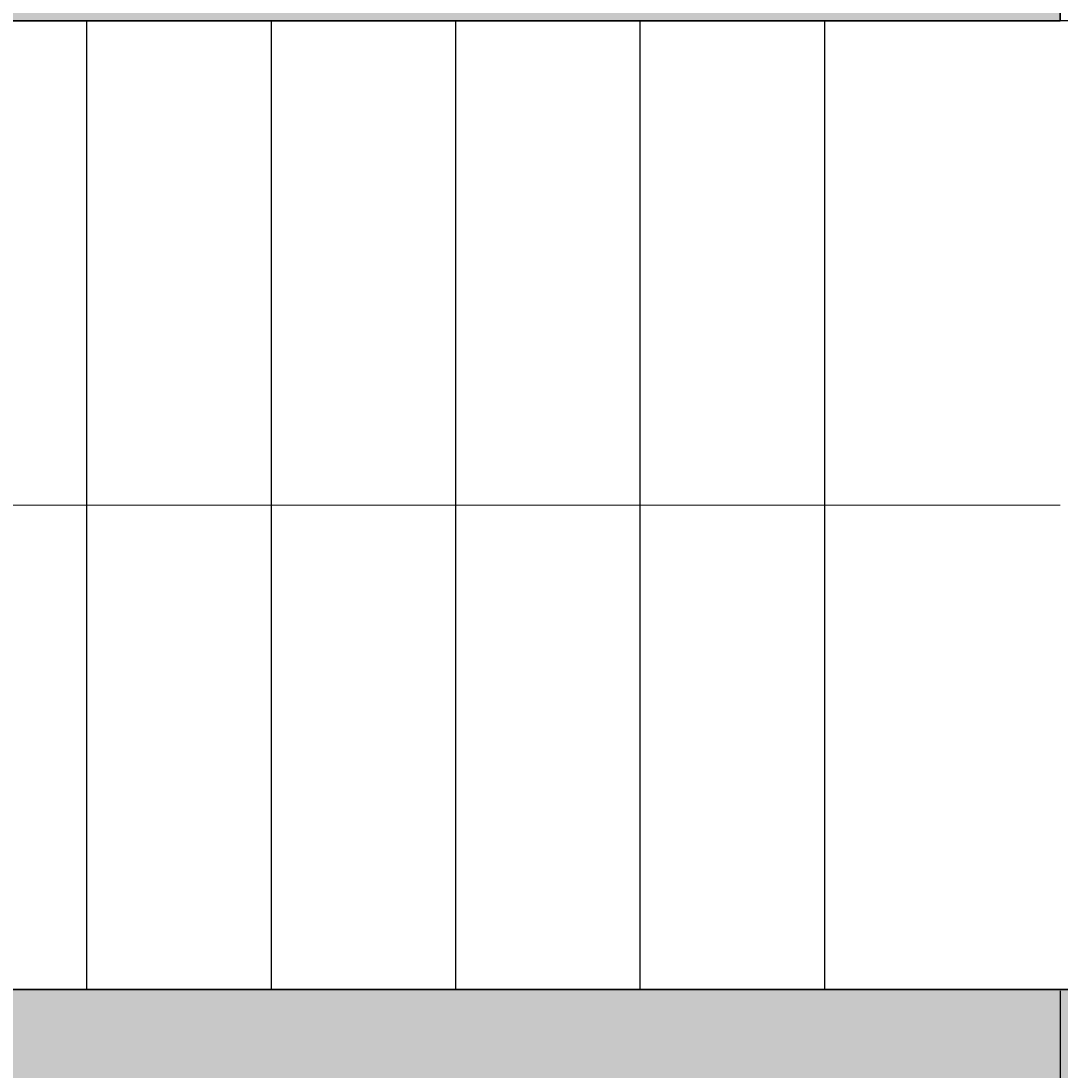
# Model space of a CAD drawing. Units: inches. Extents: x 1998 to 2588, y 1139 to 1977.
# Tile 93 of 134: x 2453 to 2498, y 1477 to 1523. Entities that reach past the tile are written whole.
import ezdxf

# ---------------------------------------------------------------- set-up
doc = ezdxf.new("R2010")
doc.units = ezdxf.units.IN
for name, color, linetype, lineweight in [('A-ANNO-DIMS', 2, 'Continuous', 18), ('A-ANNO-SYMB', 7, 'Continuous', 18), ('A-FLOR-EVTR', 7, 'Continuous', 35), ('A-FLOR-STRS', 7, 'Continuous', 25), ('A-WALL-PATT', 252, 'Continuous', 13), ('WALL', 200, 'Continuous', 35)]:
    doc.layers.add(name, color=color, linetype=linetype, lineweight=lineweight)
doc.styles.get("Standard").update_dxf_attribs({"font": 'arial.ttf'})
doc.dimstyles.get("Standard").update_dxf_attribs({"dimtxt": 0.18, "dimasz": 0.18, "dimexe": 0.18, "dimexo": 0.0625, "dimgap": 0.09, "dimtad": 0, "dimtih": 1, "dimtoh": 1, "dimdec": 4, "dimzin": 0, "dimdsep": 46, "dimtxsty": 'Standard', "dimcen": 0.09, "dimadec": 0, "dimazin": 0, "dimtfac": 1, "dimtdec": 4, "dimtofl": 0, "dimtmove": 0, "dimatfit": 3, "dimfxl": 1, "dimtolj": 1, "dimtzin": 0, "dimarcsym": 0})

# ---------------------------------------------------------------- blocks, each defined once
blk = doc.blocks.new('*D24')
at = {"layer": 'A-ANNO-DIMS', "color": 0, "lineweight": -2, "transparency": 16777216}
for p, q in [((2398.535, 1911.232), (2588.309, 1911.232)), ((2588.129, 1911.052), (2588.129, 1570.164)), ((2588.129, 1228.912), (2588.129, 1569.8)), ((2527.535, 1228.732), (2588.309, 1228.732))]:
    blk.add_line(p, q, dxfattribs=at)
at = {"layer": 'A-ANNO-DIMS', "color": 0, "transparency": 16777216}
for points in [[(2588.099, 1911.052), (2588.159, 1911.052), (2588.129, 1911.232)], [(2588.099, 1228.912), (2588.159, 1228.912), (2588.129, 1228.732)]]:
    blk.add_solid(points, dxfattribs=at)
at = {"layer": 'Defpoints', "color": 0, "transparency": 16777216}
for p in [(2398.473, 1911.232), (2588.129, 1911.232), (2527.473, 1228.732)]:
    blk.add_point(p, dxfattribs=at)
at = {"layer": 'A-ANNO-DIMS', "color": 0, "transparency": 16777216, "insert": (2588.129, 1569.982), "char_height": 0.18, "attachment_point": 5}
blk.add_mtext('\\A1;682.5', dxfattribs=at)
blk = doc.blocks.new('*D33')
at = {"layer": 'A-ANNO-DIMS', "color": 0, "lineweight": -2, "transparency": 16777216}
for p, q in [((2407.973, 1480.67), (2407.973, 1138.602)), ((2498.179, 1480.67), (2498.179, 1138.602)), ((2408.153, 1138.782), (2452.753, 1138.782)), ((2497.999, 1138.782), (2453.399, 1138.782))]:
    blk.add_line(p, q, dxfattribs=at)
at = {"layer": 'A-ANNO-DIMS', "color": 0, "transparency": 16777216}
for points in [[(2408.153, 1138.812), (2408.153, 1138.752), (2407.973, 1138.782)], [(2497.999, 1138.812), (2497.999, 1138.752), (2498.179, 1138.782)]]:
    blk.add_solid(points, dxfattribs=at)
at = {"layer": 'Defpoints', "color": 0, "transparency": 16777216}
for p in [(2407.973, 1480.732), (2498.179, 1480.732), (2498.179, 1138.782)]:
    blk.add_point(p, dxfattribs=at)
at = {"layer": 'A-ANNO-DIMS', "color": 0, "transparency": 16777216, "insert": (2453.076, 1138.782), "char_height": 0.18, "attachment_point": 5}
blk.add_mtext('\\A1;90.2', dxfattribs=at)

msp = doc.modelspace()

# ---------------------------------------------------------------- hatches: boundary and pattern name
at = {"layer": 'A-WALL-PATT'}
h = msp.add_hatch(color=256, dxfattribs=at)
h.dxf.hatch_style = 1
h.paths.add_polyline_path([(2527.4729, 1362.2324), (2510.9729, 1362.2324), (2510.9729, 1357.7324), (2518.4729, 1357.7324), (2518.4729, 1237.7324), (2503.1458, 1237.7324), (2503.1458, 1228.7324), (2527.4729, 1228.7324)])
h.paths.add_polyline_path([(2490.5682, 1362.2324), (2398.4729, 1362.2324), (2398.4729, 1357.7324), (2490.5682, 1357.7324)])
h.paths.add_polyline_path([(2224.9729, 1264.7324), (2222.9729, 1264.7324), (2222.9729, 1232.4125), (2341.4729, 1232.4125), (2341.4729, 1234.4125), (2224.9729, 1234.4125)])
h.paths.add_polyline_path([(2334.5332, 1273.7324), (2264.7638, 1273.7324), (2264.7638, 1269.5611, -0.043659), (2264.3413, 1264.7324), (2334.5332, 1264.7324)])
h.paths.add_polyline_path([(2236.9551, 1273.7324), (2234.4125, 1273.7324), (2234.4125, 1264.7324), (2236.9551, 1264.7324), (2236.9551, 1269.5611)])
h.paths.add_polyline_path([(2222.9729, 1293.2324), (2096.9729, 1293.2324), (2096.9729, 1345.0966), (2087.9729, 1345.0966), (2087.9729, 1284.2324), (2222.9729, 1284.2324), (2222.9729, 1285.137)])
h.paths.add_polyline_path([(2096.9729, 1458.7927), (2087.9729, 1458.7927), (2087.9729, 1417.7324), (2087.9729, 1413.2324), (2096.9729, 1413.2324), (2096.9729, 1417.7324)])
h.paths.add_polyline_path([(2096.9729, 1413.2324), (2087.9729, 1413.2324), (2087.9729, 1365.5012), (2096.9729, 1365.5012), (2096.9729, 1369.3358)])
h.paths.add_polyline_path([(2186.2943, 1417.7324), (2138.6074, 1417.7324), (2096.9729, 1417.7324), (2096.9729, 1413.2324), (2138.6074, 1413.2324), (2186.2943, 1413.2324)])
h.paths.add_polyline_path([(2181.4729, 1465.7324), (2176.9729, 1465.7324), (2176.9729, 1451.6434), (2181.4729, 1451.6434)])
h.paths.add_polyline_path([(2181.4729, 1422.1664), (2176.9729, 1422.1664), (2176.9729, 1417.7324), (2181.4729, 1417.7324)])
h.paths.add_polyline_path([(2063.9729, 1465.7324), (2087.9729, 1465.7324), (2087.9729, 1470.2324), (2059.4729, 1470.2324), (2059.4729, 1413.2324), (2087.9729, 1413.2324), (2087.9729, 1417.7324), (2063.9729, 1417.7324)])
h.paths.add_polyline_path([(2181.4729, 1755.2324), (2176.9729, 1755.2324), (2176.9729, 1748.6798), (2177.0513, 1748.6798), (2181.4729, 1748.6798)])
h.paths.add_polyline_path([(2227.4729, 1707.2324), (2220.4647, 1707.2324), (2220.4647, 1702.7324), (2222.9729, 1702.7324), (2222.9729, 1604.637), (2227.4729, 1604.637)])
h.paths.add_polyline_path([(2114.9729, 1702.7324), (2105.9729, 1702.7324), (2105.9729, 1628.4781, -0.0318759), (2110.1012, 1628.7416), (2114.9729, 1628.7416)])
h.paths.add_polyline_path([(2345.9729, 1739.3278), (2341.4729, 1739.3278), (2341.4729, 1647.5211), (2345.9729, 1647.5211)])
h.paths.add_polyline_path([(2350.6273, 1641.2324), (2345.9729, 1641.2324), (2345.9729, 1636.7324), (2350.6273, 1636.7324), (2350.6273, 1639.8729)])
h.paths.add_polyline_path([(2501.9729, 1641.2324), (2407.9729, 1641.2324), (2392.5005, 1641.2324), (2392.5005, 1639.8729), (2392.5005, 1636.7324), (2501.9729, 1636.7324)])
h.paths.add_polyline_path([(2510.9729, 1755.2324), (2501.9729, 1755.2324), (2501.9729, 1641.2324), (2510.9729, 1641.2324)])
h.paths.add_polyline_path([(2549.1786, 1641.2324), (2522.3775, 1641.2324), (2522.3775, 1636.7324), (2540.1786, 1636.7324), (2540.1786, 1480.7324), (2522.3775, 1480.7324), (2522.3775, 1476.2324), (2549.1786, 1476.2324)])
h.paths.add_polyline_path([(2498.1786, 1594.7324), (2407.9729, 1594.7324), (2407.9729, 1585.7324), (2416.9729, 1585.7324), (2489.1786, 1585.7324), (2489.1786, 1531.7324), (2416.9729, 1531.7324), (2407.9729, 1531.7324), (2407.9729, 1522.7324), (2498.1786, 1522.7324)])
h.paths.add_polyline_path([(2351.6437, 1480.7324), (2345.9729, 1480.7324), (2345.9729, 1476.2324), (2351.6437, 1476.2324), (2351.6437, 1477.5919)])
h.paths.add_polyline_path([(2501.9729, 1480.7324), (2498.1786, 1480.7324), (2407.9729, 1480.7324), (2393.5168, 1480.7324), (2393.5168, 1477.5919), (2393.5168, 1476.2324), (2501.9729, 1476.2324)])

# ---------------------------------------------------------------- linework, layer by layer
at = {"layer": 'A-ANNO-SYMB'}
msp.add_line((2407.9729, 1501.7324), (2498.1786, 1501.7324), dxfattribs=at)
at = {"layer": 'A-FLOR-EVTR'}
msp.add_lwpolyline([(2407.9729, 1522.7324), (2498.1786, 1522.7324), (2498.1786, 1594.7324), (2407.9729, 1594.7324)], close=True, dxfattribs=at)
at = {"layer": 'A-FLOR-STRS'}
for p, q in [((2540.1786, 1522.7324), (2407.9729, 1522.7324)), ((2455.9729, 1480.7324), (2455.9729, 1522.7324)), ((2463.9729, 1480.7324), (2463.9729, 1522.7324)), ((2471.9729, 1480.7324), (2471.9729, 1522.7324)), ((2479.9729, 1480.7324), (2479.9729, 1522.7324)), ((2487.9729, 1480.7324), (2487.9729, 1522.7324))]:
    msp.add_line(p, q, dxfattribs=at)
at = {"layer": 'WALL'}
msp.add_line((2540.1786, 1480.7324), (2407.9729, 1480.7324), dxfattribs=at)

# ---------------------------------------------------------------- dimensions: what is measured, and where the dimension line sits
at = {"layer": 'A-ANNO-DIMS'}
dim = msp.add_linear_dim(base=(2588.1286, 1911.2324), p1=(2527.4729, 1228.7324), p2=(2398.4729, 1911.2324), angle=90, dimstyle='Standard', override={"dimdec": 1, "dimlfac": 1, "dimrnd": 0, "dimzin": 0, "dimdsep": 46, "dimlunit": 2}, dxfattribs=at)
dim.commit()
dim.dimension.update_dxf_attribs({"geometry": '*D24', "text_midpoint": (2588.1286, 1569.9824)})
dim = msp.add_linear_dim(base=(2498.1786, 1138.7824), p1=(2407.9729, 1480.7324), p2=(2498.1786, 1480.7324), dimstyle='Standard', override={"dimdec": 1, "dimlfac": 1, "dimrnd": 0, "dimzin": 0, "dimdsep": 46, "dimlunit": 2}, dxfattribs=at)
dim.commit()
dim.dimension.update_dxf_attribs({"geometry": '*D33', "text_midpoint": (2453.0757, 1138.7824)})

doc.saveas('drawing.dxf')
